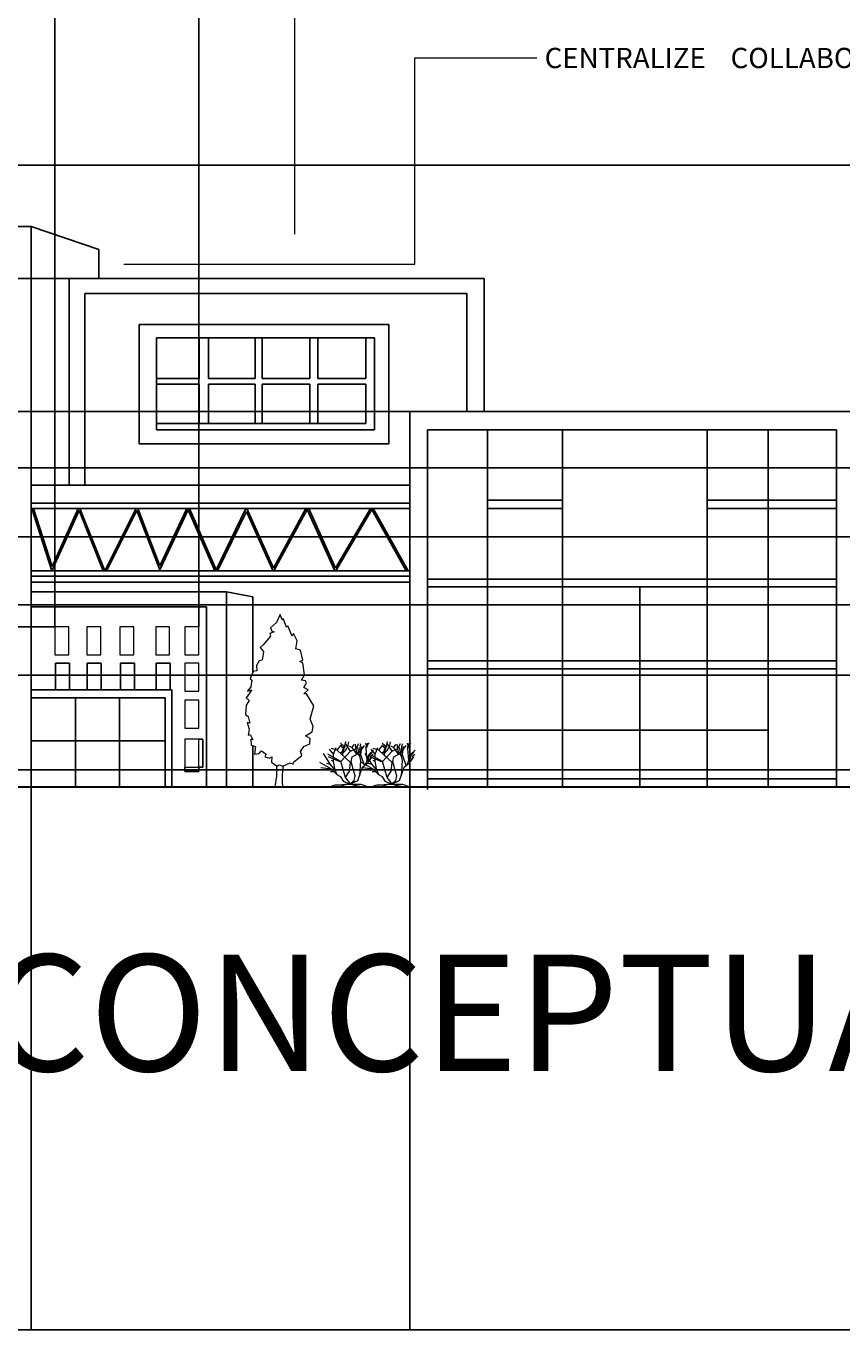
# Model space of a CAD drawing. Units: inches. Extents: x -32109 to 33221, y -19197 to 7608.
# Tile 12 of 25: x -5707 to -741, y -5430 to 2510. Entities that reach past the tile are written whole.
import ezdxf

# ---------------------------------------------------------------- set-up
doc = ezdxf.new("R2010")
doc.units = ezdxf.units.IN
doc.header["$MEASUREMENT"] = 0
for name, color, linetype, lineweight in [('A-ANNO-DIMS', 2, 'Continuous', 18), ('A-ANNO-NOTE', 2, 'Continuous', 18), ('A-ANNO-TEXT', 7, 'Continuous', 25), ('A-ELEV', 7, 'Continuous', 25), ('A-GLAZ', 4, 'Continuous', 18), ('L-PLNT', 3, 'Continuous', 13)]:
    doc.layers.add(name, color=color, linetype=linetype, lineweight=lineweight)
doc.styles.get("Standard").update_dxf_attribs({"font": 'arial.ttf'})
doc.dimstyles.get("Standard").update_dxf_attribs({"dimtxt": 0.18, "dimasz": 0.18, "dimexe": 0.18, "dimexo": 0.0625, "dimgap": 0.09, "dimtad": 0, "dimtih": 1, "dimtoh": 1, "dimdec": 4, "dimzin": 0, "dimdsep": 46, "dimtxsty": 'Standard', "dimcen": 0.09, "dimadec": 0, "dimazin": 0, "dimtfac": 1, "dimtdec": 4, "dimtofl": 0, "dimtmove": 0, "dimatfit": 3, "dimfxl": 1, "dimtolj": 1, "dimtzin": 0, "dimarcsym": 0})

# ---------------------------------------------------------------- blocks, each defined once
blk = doc.blocks.new('*U2')
blk.add_lwpolyline([(-2.754, 191.699), (-6.78, 182.851), (-13.682, 176.953), (-11.956, 173.266), (-9.656, 172.529), (-14.257, 170.317), (-13.682, 167.368), (-21.733, 157.783), (-25.184, 154.834), (-21.158, 150.41), (-21.733, 147.461), (-22.884, 140.825), (-26.334, 140.087), (-29.21, 134.926), (-28.635, 129.028), (-32.661, 128.291), (-36.111, 120.18), (-34.386, 118.706), (-35.536, 111.333), (-38.987, 106.171), (-34.386, 107.646), (-40.712, 98.798), (-37.261, 95.849), (-40.712, 90.688), (-41.287, 80.366), (-38.412, 78.154), (-36.686, 70.781), (-39.562, 71.518), (-37.261, 64.145), (-38.412, 57.509), (-36.111, 58.247), (-33.236, 52.348), (-35.536, 53.086), (-34.961, 46.45), (-30.36, 44.975), (-31.51, 36.128), (-26.334, 36.865), (-23.459, 39.814), (-18.283, 36.128), (-20.008, 33.178), (-14.832, 31.704), (-11.956, 33.178), (-12.531, 27.28), (-6.205, 22.856), (-3.905, 24.331), (0.121, 22.856), (8.173, 26.543), (11.624, 25.068), (12.199, 27.28), (21.4, 34.653), (19.675, 39.077), (23.701, 44.975), (30.027, 47.924), (30.602, 53.823), (25.426, 56.772), (32.903, 61.196), (34.053, 67.094), (30.602, 75.205), (34.628, 89.951), (26.576, 103.222), (23.701, 103.222), (28.302, 107.646), (23.701, 110.595), (26.576, 115.756), (25.426, 117.968), (20.825, 118.706), (24.276, 124.604), (22.551, 137.876), (19.1, 139.35), (22.551, 140.825), (19.675, 151.884), (14.499, 153.359), (16.224, 162.207), (12.199, 170.317), (10.473, 167.368), (5.872, 179.165), (4.147, 177.69), (0.696, 187.275), (-0.454, 185.8)], close=True)
for points in [[(-6.813, 23.669), (-6.813, 11.669), (-8.627, 0)], [(0.387, 23.669), (-0.576, 13.271), (-0.576, 3.686), (0, 0)]]:
    blk.add_lwpolyline(points)
blk = doc.blocks.new('*U3')
for p, q in [((-14.88, 18.24), (-12.96, 20.64)), ((-12.471, 19.775), (-12.898, 22.044)), ((-11.28, 19.619), (-12.104, 21.184)), ((-11.921, 18.836), (-10.64, 20.401)), ((-11.433, 18.289), (-10.457, 22.749)), ((-8.16, 17.76), (-10.56, 21.6)), ((-9.48, 19.775), (-8.992, 22.592)), ((-7.2, 19.68), (-8.64, 20.16)), ((-7.2, 19.68), (-6.24, 21.12)), ((-5.086, 17.741), (-5.513, 21.34)), ((-5.28, 19.2), (-3.84, 21.6)), ((-3.84, 16.8), (-0.96, 20.64)), ((-3.377, 18.602), (-2.888, 21.575)), ((-2.88, 15.84), (-2.4, 20.16)), ((-0.508, 21.888), (-0.081, 20.558)), ((-0.203, 19.149), (0.102, 21.34)), ((-0.142, 19.384), (0.59, 20.401)), ((-0.02, 20.01), (0.896, 21.105)), ((0.041, 20.714), (1.384, 22.044)), ((0.102, 21.34), (0.835, 21.888)), ((-18.24, 11.04), (-21.755, 16.655)), ((-12.96, 12.48), (-19.68, 16.32)), ((-13.92, 12.48), (-19.2, 14.88)), ((-16.8, 16.32), (-18.72, 18.72)), ((-14.88, 18.24), (-17.76, 19.2)), ((-16.8, 16.32), (-15.36, 19.68)), ((-16.8, 12.48), (-16.8, 16.32)), ((-8.16, 12), (-14.88, 18.24)), ((-13.325, 16.724), (-11.433, 18.289)), ((-12.96, 12.48), (-8.16, 17.76)), ((-11.677, 19.071), (-12.471, 19.775)), ((-12.043, 15.628), (-11.921, 18.836)), ((-11.982, 16.802), (-10.579, 18.054)), ((-10.579, 18.054), (-9.846, 19.697)), ((-8.16, 17.76), (-5.28, 19.2)), ((-7.68, 12.48), (-7.2, 14.88)), ((-4.8, 16.32), (-7.2, 19.68)), ((-7.2, 14.88), (-3.84, 16.8)), ((-3.377, 15.315), (-5.086, 17.819)), ((-2.88, 12.96), (-4.32, 19.68)), ((-2.766, 16.802), (-3.377, 18.602)), ((-0.96, 10.56), (-2.88, 15.84)), ((0.346, 13.203), (-0.203, 19.149)), ((0.346, 13.203), (1.323, 16.254)), ((0.96, 12), (1.44, 15.36)), ((0.96, 12), (2.88, 14.88)), ((1.323, 16.254), (3.642, 18.289)), ((1.44, 15.36), (2.88, 17.28)), ((1.92, 13.44), (2.4, 15.36)), ((2.4, 15.36), (3.36, 16.32)), ((-17.76, 8.64), (-23.663, 11.961)), ((-17.76, 8.64), (-23.128, 9.222)), ((-18.24, 11.04), (-20.16, 11.52)), ((-15.84, 8.16), (-18.24, 11.04)), ((-16.32, 7.2), (-18.24, 7.2)), ((-16.8, 12.48), (-17.76, 12.96)), ((-14.88, 5.76), (-17.76, 8.64)), ((-15.84, 8.16), (-16.8, 12.48)), ((-14.88, 5.76), (-15.84, 8.16)), ((-12.96, 12.48), (-13.92, 12.48)), ((-10.56, 4.32), (-12.96, 12.48)), ((-10.56, 4.32), (-8.64, 7.68)), ((-8.64, 7.68), (-8.16, 12)), ((-6.72, 8.64), (-7.68, 12.48)), ((-5.76, 5.28), (-6.72, 8.64)), ((-4.32, 2.88), (-1.92, 9.6)), ((-3.36, 5.28), (-2.88, 12.96)), ((-1.92, 9.6), (0.96, 12)), ((-0.48, 10.8), (0.346, 13.203)), ((-15.84, 0.48), (-17.76, 0)), ((-13.44, 0.48), (-15.84, 0.48)), ((-12.96, 4.8), (-14.88, 5.76)), ((-9.6, 0.96), (-13.44, 0.48)), ((-11.52, 2.4), (-12.96, 4.8)), ((-9.6, 0.96), (-12.96, 0)), ((-8.64, 0.96), (-11.52, 2.4)), ((-8.64, 1.92), (-10.56, 4.32)), ((-9.6, 0.96), (-7.68, 0.96)), ((-8.64, 0.96), (-4.32, 2.88)), ((-8.64, 0.96), (-6.24, 2.88)), ((-8.64, 0.96), (-8.64, 1.92)), ((-8.64, 0.96), (-2.88, 0.96)), ((-7.68, 0.96), (-6.24, 0.48)), ((-6.24, 2.88), (-5.76, 5.28)), ((-6.24, 0.48), (-3.36, 0)), ((-2.88, 0.96), (0, 0))]:
    blk.add_line(p, q)
blk = doc.blocks.new('WIN-SMALL-A')
for p, q in [((0, 169.6), (0, 0)), ((84.9, 169.6), (0, 169.6)), ((84.9, 0), (84.9, 169.6)), ((0, 0), (84.9, 0))]:
    blk.add_line(p, q)
blk = doc.blocks.new('*D6')
at = {"layer": 'A-ANNO-DIMS', "color": 0, "lineweight": -2, "transparency": 16777216}
for p, q in [((-4656.1, -1833.3), (-4630.5, -1833.3)), ((-4630.7, -1833.5), (-4630.7, -1917.9)), ((-4630.7, -2002.8), (-4630.7, -1918.3)), ((-4656.1, -2002.9), (-4630.5, -2002.9))]:
    blk.add_line(p, q, dxfattribs=at)
at = {"layer": 'A-ANNO-DIMS', "color": 0, "transparency": 16777216}
for points in [[(-4630.7, -1833.5), (-4630.7, -1833.5), (-4630.7, -1833.3)], [(-4630.7, -2002.8), (-4630.7, -2002.8), (-4630.7, -2002.9)]]:
    blk.add_solid(points, dxfattribs=at)
at = {"layer": 'Defpoints', "color": 0, "transparency": 16777216}
for p in [(-4656.1, -1833.3), (-4656.1, -2002.9), (-4630.7, -2002.9)]:
    blk.add_point(p, dxfattribs=at)
at = {"layer": 'A-ANNO-DIMS', "color": 0, "transparency": 16777216, "insert": (-4630.7, -1918.1), "char_height": 0.18, "attachment_point": 5}
blk.add_mtext('\\A1;SMALL WINDOW A 170 TYP.', dxfattribs=at)
blk = doc.blocks.new('*D7')
at = {"layer": 'A-ANNO-DIMS', "color": 0, "lineweight": -2, "transparency": 16777216}
for p, q in [((-4741.1, -2003), (-4741.1, -2028.6)), ((-4740.9, -2028.4), (-4699.1, -2028.4)), ((-4656.3, -2028.4), (-4698.1, -2028.4)), ((-4656.1, -2003), (-4656.1, -2028.6))]:
    blk.add_line(p, q, dxfattribs=at)
at = {"layer": 'A-ANNO-DIMS', "color": 0, "transparency": 16777216}
for points in [[(-4740.9, -2028.4), (-4740.9, -2028.4), (-4741.1, -2028.4)], [(-4656.3, -2028.4), (-4656.3, -2028.4), (-4656.1, -2028.4)]]:
    blk.add_solid(points, dxfattribs=at)
at = {"layer": 'Defpoints', "color": 0, "transparency": 16777216}
for p in [(-4741.1, -2002.9), (-4741.1, -2028.4), (-4656.1, -2002.9)]:
    blk.add_point(p, dxfattribs=at)
at = {"layer": 'A-ANNO-DIMS', "color": 0, "transparency": 16777216, "insert": (-4698.6, -2028.4), "char_height": 0.18, "attachment_point": 5}
blk.add_mtext('\\A1;85 TYP.', dxfattribs=at)
blk = doc.blocks.new('*D10')
at = {"layer": 'A-ANNO-DIMS', "color": 0, "lineweight": -2, "transparency": 16777216}
for p, q in [((-18512.6, -110.2), (-18512.6, 5772)), ((-18512.5, 5771.8), (-202.1, 5771.8)), ((18109.1, 5771.8), (-201.2, 5771.8)), ((18109.3, -101.5), (18109.3, 5772))]:
    blk.add_line(p, q, dxfattribs=at)
at = {"layer": 'A-ANNO-DIMS', "color": 0, "transparency": 16777216}
for points in [[(-18512.5, 5771.9), (-18512.5, 5771.8), (-18512.6, 5771.8)], [(18109.1, 5771.9), (18109.1, 5771.8), (18109.3, 5771.8)]]:
    blk.add_solid(points, dxfattribs=at)
at = {"layer": 'Defpoints', "color": 0, "transparency": 16777216}
for p in [(18109.3, 5771.8), (-18512.6, -110.2), (18109.3, -101.6)]:
    blk.add_point(p, dxfattribs=at)
at = {"layer": 'A-ANNO-DIMS', "color": 0, "transparency": 16777216, "insert": (-201.7, 5771.8), "char_height": 0.18, "attachment_point": 5}
blk.add_mtext('\\A1;36622', dxfattribs=at)
blk = doc.blocks.new('*D11')
at = {"layer": 'A-ANNO-DIMS', "color": 0, "lineweight": -2, "transparency": 16777216}
for p, q in [((14509.6, 1705.2), (25710.6, 1705.2)), ((25710.5, 1705), (25710.5, -209.6)), ((25710.5, -2124.6), (25710.5, -210)), ((-18512.6, -2124.8), (25710.6, -2124.8))]:
    blk.add_line(p, q, dxfattribs=at)
at = {"layer": 'A-ANNO-DIMS', "color": 0, "transparency": 16777216}
for points in [[(25710.4, 1705), (25710.5, 1705), (25710.5, 1705.2)], [(25710.4, -2124.6), (25710.5, -2124.6), (25710.5, -2124.8)]]:
    blk.add_solid(points, dxfattribs=at)
at = {"layer": 'Defpoints', "color": 0, "transparency": 16777216}
for p in [(14509.6, 1705.2), (-18512.6, -2124.8), (25710.5, -2124.8)]:
    blk.add_point(p, dxfattribs=at)
at = {"layer": 'A-ANNO-DIMS', "color": 0, "transparency": 16777216, "insert": (25710.5, -209.8), "char_height": 0.18, "attachment_point": 5}
blk.add_mtext('\\A1;3830', dxfattribs=at)
blk = doc.blocks.new('*D20')
at = {"layer": 'A-ANNO-DIMS', "color": 0, "lineweight": -2, "transparency": 16777216}
for p, q in [((-5532.1, -1149.2), (-5532.1, 5772)), ((-5531.9, 5771.8), (-5094.4, 5771.8)), ((-4656.3, 5771.8), (-5093.8, 5771.8)), ((-4656.1, -1149.2), (-4656.1, 5772))]:
    blk.add_line(p, q, dxfattribs=at)
at = {"layer": 'A-ANNO-DIMS', "color": 0, "transparency": 16777216}
for points in [[(-5531.9, 5771.9), (-5531.9, 5771.8), (-5532.1, 5771.8)], [(-4656.3, 5771.9), (-4656.3, 5771.8), (-4656.1, 5771.8)]]:
    blk.add_solid(points, dxfattribs=at)
at = {"layer": 'Defpoints', "color": 0, "transparency": 16777216}
for p in [(-4656.1, 5771.8), (-5532.1, -1149.2), (-4656.1, -1149.2)]:
    blk.add_point(p, dxfattribs=at)
at = {"layer": 'A-ANNO-DIMS', "color": 0, "transparency": 16777216, "insert": (-5094.1, 5771.8), "char_height": 0.18, "attachment_point": 5}
blk.add_mtext('\\A1;876', dxfattribs=at)
blk = doc.blocks.new('*D21')
at = {"layer": 'A-ANNO-DIMS', "color": 0, "lineweight": -2, "transparency": 16777216}
for p, q in [((-5532.2, -1149.2), (-24362, -1149.2)), ((-24361.8, -1149.4), (-24361.8, -1636.8)), ((-24361.8, -2124.6), (-24361.8, -1637.2)), ((-5677.1, -2124.8), (-24362, -2124.8))]:
    blk.add_line(p, q, dxfattribs=at)
at = {"layer": 'A-ANNO-DIMS', "color": 0, "transparency": 16777216}
for points in [[(-24361.8, -1149.4), (-24361.8, -1149.4), (-24361.8, -1149.2)], [(-24361.8, -2124.6), (-24361.8, -2124.6), (-24361.8, -2124.8)]]:
    blk.add_solid(points, dxfattribs=at)
at = {"layer": 'Defpoints', "color": 0, "transparency": 16777216}
for p in [(-24361.8, -1149.2), (-5532.1, -1149.2), (-5677.1, -2124.8)]:
    blk.add_point(p, dxfattribs=at)
at = {"layer": 'A-ANNO-DIMS', "color": 0, "transparency": 16777216, "insert": (-24361.8, -1637), "char_height": 0.18, "attachment_point": 5}
blk.add_mtext('\\A1;975.6', dxfattribs=at)
blk = doc.blocks.new('*D29')
at = {"layer": 'A-ANNO-DIMS', "color": 0, "lineweight": -2, "transparency": 16777216}
for p, q in [((-7754.4, -2118.5), (-7754.4, -5429.7)), ((-5677.1, -2124.9), (-5677.1, -5429.7)), ((-7754.2, -5429.6), (-6716.2, -5429.6)), ((-5677.3, -5429.6), (-6715.3, -5429.6))]:
    blk.add_line(p, q, dxfattribs=at)
at = {"layer": 'A-ANNO-DIMS', "color": 0, "transparency": 16777216}
for points in [[(-7754.2, -5429.5), (-7754.2, -5429.6), (-7754.4, -5429.6)], [(-5677.3, -5429.5), (-5677.3, -5429.6), (-5677.1, -5429.6)]]:
    blk.add_solid(points, dxfattribs=at)
at = {"layer": 'Defpoints', "color": 0, "transparency": 16777216}
for p in [(-7754.4, -2118.4), (-5677.1, -2124.8), (-5677.1, -5429.6)]:
    blk.add_point(p, dxfattribs=at)
at = {"layer": 'A-ANNO-DIMS', "color": 0, "transparency": 16777216, "insert": (-6715.7, -5429.6), "char_height": 0.18, "attachment_point": 5}
blk.add_mtext('\\A1;2077.3', dxfattribs=at)
blk = doc.blocks.new('*D30')
at = {"layer": 'A-ANNO-DIMS', "color": 0, "lineweight": -2, "transparency": 16777216}
for p, q in [((-5677.1, -2124.9), (-5677.1, -5429.7)), ((-3370.6, -2124.9), (-3370.6, -5429.7)), ((-5676.9, -5429.6), (-4524.3, -5429.6)), ((-3370.7, -5429.6), (-4523.4, -5429.6))]:
    blk.add_line(p, q, dxfattribs=at)
at = {"layer": 'A-ANNO-DIMS', "color": 0, "transparency": 16777216}
for points in [[(-5676.9, -5429.5), (-5676.9, -5429.6), (-5677.1, -5429.6)], [(-3370.7, -5429.5), (-3370.7, -5429.6), (-3370.6, -5429.6)]]:
    blk.add_solid(points, dxfattribs=at)
at = {"layer": 'Defpoints', "color": 0, "transparency": 16777216}
for p in [(-5677.1, -2124.8), (-3370.6, -2124.8), (-3370.6, -5429.6)]:
    blk.add_point(p, dxfattribs=at)
at = {"layer": 'A-ANNO-DIMS', "color": 0, "transparency": 16777216, "insert": (-4523.8, -5429.6), "char_height": 0.18, "attachment_point": 5}
blk.add_mtext('\\A1;2306.5', dxfattribs=at)
blk = doc.blocks.new('*D31')
at = {"layer": 'A-ANNO-DIMS', "color": 0, "lineweight": -2, "transparency": 16777216}
for p, q in [((-3370.6, -2124.9), (-3370.6, -5429.7)), ((-651, -2124.9), (-651, -5429.7)), ((-3370.4, -5429.6), (-2011.2, -5429.6)), ((-651.1, -5429.6), (-2010.3, -5429.6))]:
    blk.add_line(p, q, dxfattribs=at)
at = {"layer": 'A-ANNO-DIMS', "color": 0, "transparency": 16777216}
for points in [[(-3370.4, -5429.5), (-3370.4, -5429.6), (-3370.6, -5429.6)], [(-651.1, -5429.5), (-651.1, -5429.6), (-651, -5429.6)]]:
    blk.add_solid(points, dxfattribs=at)
at = {"layer": 'Defpoints', "color": 0, "transparency": 16777216}
for p in [(-3370.6, -2124.8), (-651, -2124.8), (-651, -5429.6)]:
    blk.add_point(p, dxfattribs=at)
at = {"layer": 'A-ANNO-DIMS', "color": 0, "transparency": 16777216, "insert": (-2010.8, -5429.6), "char_height": 0.18, "attachment_point": 5}
blk.add_mtext('\\A1;2719.6', dxfattribs=at)
blk = doc.blocks.new('*D40')
at = {"layer": 'A-ANNO-DIMS', "color": 0, "lineweight": -2, "transparency": 16777216}
for p, q in [((-5445.1, 973), (-24362, 973)), ((-24361.8, 972.8), (-24361.8, -575.7)), ((-24361.8, -2124.6), (-24361.8, -576.1)), ((-5677.1, -2124.8), (-24362, -2124.8))]:
    blk.add_line(p, q, dxfattribs=at)
at = {"layer": 'A-ANNO-DIMS', "color": 0, "transparency": 16777216}
for points in [[(-24361.8, 972.8), (-24361.8, 972.8), (-24361.8, 973)], [(-24361.8, -2124.6), (-24361.8, -2124.6), (-24361.8, -2124.8)]]:
    blk.add_solid(points, dxfattribs=at)
at = {"layer": 'Defpoints', "color": 0, "transparency": 16777216}
for p in [(-5445, 973), (-24361.8, -2124.8), (-5677.1, -2124.8)]:
    blk.add_point(p, dxfattribs=at)
at = {"layer": 'A-ANNO-DIMS', "color": 0, "transparency": 16777216, "insert": (-24361.8, -575.9), "char_height": 0.18, "attachment_point": 5}
blk.add_mtext('\\A1;3098', dxfattribs=at)
blk = doc.blocks.new('*D41')
at = {"layer": 'A-ANNO-DIMS', "color": 0, "lineweight": -2, "transparency": 16777216}
for p, q in [((-651, 162.2), (-24362, 162.2)), ((-24361.8, 162), (-24361.8, -981.1)), ((-24361.8, -2124.6), (-24361.8, -981.5)), ((-651, -2124.8), (-24362, -2124.8))]:
    blk.add_line(p, q, dxfattribs=at)
at = {"layer": 'A-ANNO-DIMS', "color": 0, "transparency": 16777216}
for points in [[(-24361.8, 162), (-24361.8, 162), (-24361.8, 162.2)], [(-24361.8, -2124.6), (-24361.8, -2124.6), (-24361.8, -2124.8)]]:
    blk.add_solid(points, dxfattribs=at)
at = {"layer": 'Defpoints', "color": 0, "transparency": 16777216}
for p in [(-651, 162.2), (-24361.8, -2124.8), (-651, -2124.8)]:
    blk.add_point(p, dxfattribs=at)
at = {"layer": 'A-ANNO-DIMS', "color": 0, "transparency": 16777216, "insert": (-24361.8, -981.3), "char_height": 0.18, "attachment_point": 5}
blk.add_mtext('\\A1;2287', dxfattribs=at)
blk = doc.blocks.new('*D53')
at = {"layer": 'A-ANNO-DIMS', "color": 0, "lineweight": -2, "transparency": 16777216}
for p, q in [((-9508.3, -179.7), (25710.6, -179.7)), ((25710.5, -179.9), (25710.5, -389.7)), ((25710.5, -600), (25710.5, -390.1)), ((-9508.3, -600.2), (25710.6, -600.2))]:
    blk.add_line(p, q, dxfattribs=at)
at = {"layer": 'A-ANNO-DIMS', "color": 0, "transparency": 16777216}
for points in [[(25710.4, -179.9), (25710.5, -179.9), (25710.5, -179.7)], [(25710.4, -600), (25710.5, -600), (25710.5, -600.2)]]:
    blk.add_solid(points, dxfattribs=at)
at = {"layer": 'Defpoints', "color": 0, "transparency": 16777216}
for p in [(-9508.3, -179.7), (-9508.3, -600.2), (25710.5, -600.2)]:
    blk.add_point(p, dxfattribs=at)
at = {"layer": 'A-ANNO-DIMS', "color": 0, "transparency": 16777216, "insert": (25710.5, -389.9), "char_height": 0.18, "attachment_point": 5}
blk.add_mtext('\\A1;420.5', dxfattribs=at)
blk = doc.blocks.new('*D54')
at = {"layer": 'A-ANNO-DIMS', "color": 0, "lineweight": -2, "transparency": 16777216}
for p, q in [((-9508.3, -600.2), (25710.6, -600.2)), ((25710.5, -600.3), (25710.5, -806.8)), ((25710.5, -1013.7), (25710.5, -807.2)), ((-9508.3, -1013.9), (25710.6, -1013.9))]:
    blk.add_line(p, q, dxfattribs=at)
at = {"layer": 'A-ANNO-DIMS', "color": 0, "transparency": 16777216}
for points in [[(25710.4, -600.3), (25710.5, -600.3), (25710.5, -600.2)], [(25710.4, -1013.7), (25710.5, -1013.7), (25710.5, -1013.9)]]:
    blk.add_solid(points, dxfattribs=at)
at = {"layer": 'Defpoints', "color": 0, "transparency": 16777216}
for p in [(-9508.3, -600.2), (-9508.3, -1013.9), (25710.5, -1013.9)]:
    blk.add_point(p, dxfattribs=at)
at = {"layer": 'A-ANNO-DIMS', "color": 0, "transparency": 16777216, "insert": (25710.5, -807), "char_height": 0.18, "attachment_point": 5}
blk.add_mtext('\\A1;413.7', dxfattribs=at)
blk = doc.blocks.new('*D55')
at = {"layer": 'A-ANNO-DIMS', "color": 0, "lineweight": -2, "transparency": 16777216}
for p, q in [((-9508.3, -1013.9), (25710.6, -1013.9)), ((25710.5, -1014.1), (25710.5, -1227.7)), ((25710.5, -1441.6), (25710.5, -1228)), ((-9508.3, -1441.8), (25710.6, -1441.8))]:
    blk.add_line(p, q, dxfattribs=at)
at = {"layer": 'A-ANNO-DIMS', "color": 0, "transparency": 16777216}
for points in [[(25710.4, -1014.1), (25710.5, -1014.1), (25710.5, -1013.9)], [(25710.4, -1441.6), (25710.5, -1441.6), (25710.5, -1441.8)]]:
    blk.add_solid(points, dxfattribs=at)
at = {"layer": 'Defpoints', "color": 0, "transparency": 16777216}
for p in [(-9508.3, -1013.9), (-9508.3, -1441.8), (25710.5, -1441.8)]:
    blk.add_point(p, dxfattribs=at)
at = {"layer": 'A-ANNO-DIMS', "color": 0, "transparency": 16777216, "insert": (25710.5, -1227.9), "char_height": 0.18, "attachment_point": 5}
blk.add_mtext('\\A1;427.9', dxfattribs=at)
blk = doc.blocks.new('*D56')
at = {"layer": 'A-ANNO-DIMS', "color": 0, "lineweight": -2, "transparency": 16777216}
for p, q in [((-9508.3, -1441.8), (25710.6, -1441.8)), ((25710.5, -1442), (25710.5, -1730.1)), ((25710.5, -2018.6), (25710.5, -1730.5)), ((-9508.3, -2018.8), (25710.6, -2018.8))]:
    blk.add_line(p, q, dxfattribs=at)
at = {"layer": 'A-ANNO-DIMS', "color": 0, "transparency": 16777216}
for points in [[(25710.4, -1442), (25710.5, -1442), (25710.5, -1441.8)], [(25710.4, -2018.6), (25710.5, -2018.6), (25710.5, -2018.8)]]:
    blk.add_solid(points, dxfattribs=at)
at = {"layer": 'Defpoints', "color": 0, "transparency": 16777216}
for p in [(-9508.3, -1441.8), (-9508.3, -2018.8), (25710.5, -2018.8)]:
    blk.add_point(p, dxfattribs=at)
at = {"layer": 'A-ANNO-DIMS', "color": 0, "transparency": 16777216, "insert": (25710.5, -1730.3), "char_height": 0.18, "attachment_point": 5}
blk.add_mtext('\\A1;576.9', dxfattribs=at)
blk = doc.blocks.new('*D158')
at = {"layer": 'A-ANNO-DIMS', "color": 0, "lineweight": -2, "transparency": 16777216}
for p, q in [((5447.3, 1662.2), (-24362, 1662.2)), ((-24361.8, 1662), (-24361.8, -230.1)), ((-24361.8, -2122.6), (-24361.8, -230.5)), ((5279.2, -2122.7), (-24362, -2122.7))]:
    blk.add_line(p, q, dxfattribs=at)
at = {"layer": 'A-ANNO-DIMS', "color": 0, "transparency": 16777216}
for points in [[(-24361.8, 1662), (-24361.8, 1662), (-24361.8, 1662.2)], [(-24361.8, -2122.6), (-24361.8, -2122.6), (-24361.8, -2122.7)]]:
    blk.add_solid(points, dxfattribs=at)
at = {"layer": 'Defpoints', "color": 0, "transparency": 16777216}
for p in [(5447.3, 1662.2), (-24361.8, -2122.7), (5279.3, -2122.7)]:
    blk.add_point(p, dxfattribs=at)
at = {"layer": 'A-ANNO-DIMS', "color": 0, "transparency": 16777216, "insert": (-24361.8, -230.3), "char_height": 0.18, "attachment_point": 5}
blk.add_mtext('\\A1;3784.9', dxfattribs=at)

msp = doc.modelspace()

# ---------------------------------------------------------------- linework, layer by layer
at = {"layer": 'A-ANNO-NOTE'}
for p, q in [((-4070.256, 1242.026), (-4070.256, 3321.835)), ((-3340.327, 1059.41), (-3340.327, 2317.456)), ((-3340.327, 2317.456), (-2597.229, 2317.456)), ((-5112.618, 1059.41), (-3340.327, 1059.41))]:
    msp.add_line(p, q, dxfattribs=at)
at = {"layer": 'A-ELEV'}
for p, q in [((-5677.079, 1290.029), (-7375.878, 1290.029)), ((-5677.079, 705.707), (-5677.079, 1290.029)), ((-5677.079, 1290.029), (-5264.468, 1149.061)), ((-5264.468, 973.011), (-5264.468, 1149.061)), ((-5445.024, 973.011), (-2919.008, 973.011)), ((-5445.024, 973.011), (-5445.024, -286.113)), ((-2919.008, 973.011), (-2919.008, 162.186)), ((-5350.049, -286.113), (-5350.049, 880.414)), ((-5350.049, 880.414), (-3024.183, 880.414)), ((-3024.183, 880.414), (-3024.183, 162.186)), ((-5677.079, 705.707), (-5677.079, 115.673)), ((-5019.261, 693.125), (-3498.949, 693.125)), ((-5019.261, 693.125), (-5019.261, -33.953)), ((-3498.949, 693.125), (-3498.949, -33.953)), ((-4914.008, 611.561), (-3585.505, 611.561)), ((-4914.008, 51.166), (-4914.008, 611.561)), ((-4652.588, 364.767), (-4652.588, 611.561)), ((-4595.774, 364.767), (-4595.774, 611.561)), ((-4313.328, 364.767), (-4313.328, 611.561)), ((-4270.84, 364.767), (-4270.84, 611.561)), ((-3978.939, 364.767), (-3978.939, 611.561)), ((-3930.362, 364.767), (-3930.362, 611.561)), ((-3638.056, 364.767), (-3638.056, 611.561)), ((-3585.505, 611.561), (-3585.505, 51.166)), ((-4914.008, 364.767), (-4652.588, 364.767)), ((-4914.008, 329.958), (-4652.588, 329.958)), ((-4652.588, 90.392), (-4652.588, 329.958)), ((-4595.774, 364.767), (-4313.328, 364.767)), ((-4595.774, 90.392), (-4595.774, 329.958)), ((-4595.774, 329.958), (-4313.328, 329.958)), ((-4313.328, 90.392), (-4313.328, 329.958)), ((-4270.84, 364.767), (-3978.939, 364.767)), ((-4270.84, 90.392), (-4270.84, 329.958)), ((-4270.84, 329.958), (-3978.939, 329.958)), ((-3978.939, 90.392), (-3978.939, 329.958)), ((-3930.362, 364.767), (-3638.056, 364.767)), ((-3930.362, 90.392), (-3930.362, 329.958)), ((-3930.362, 329.958), (-3638.056, 329.958)), ((-3638.056, 90.392), (-3638.056, 329.958)), ((-3370.568, 162.186), (-3370.568, -2124.791)), ((-3370.568, 162.186), (-650.959, 162.186)), ((-5677.079, -332.626), (-5677.079, 115.673)), ((-4914.008, 90.392), (-3638.056, 90.392)), ((-3585.505, 51.166), (-4914.008, 51.166)), ((-3264.186, -2138.615), (-3264.186, 50.575)), ((-3264.186, 50.575), (-773.951, 50.575)), ((-2897.717, -2124.791), (-2897.717, 50.575)), ((-2441.631, -2124.791), (-2441.631, 50.575)), ((-1560.381, -2124.791), (-1560.381, 50.575)), ((-1189.328, -2124.791), (-1189.328, 50.575)), ((-773.951, 50.575), (-773.951, -2124.791)), ((-5019.261, -33.953), (-3498.949, -33.953)), ((-3370.568, -286.113), (-5677.079, -286.113)), ((-5677.079, -332.626), (-5677.079, -830.732)), ((-5677.079, -391.831), (-5677.079, -2124.791)), ((-3370.568, -395.582), (-5677.079, -395.582)), ((-5677.079, -428.305), (-5677.079, -395.582)), ((-2897.717, -376.671), (-2441.631, -376.671)), ((-1560.381, -376.671), (-773.951, -376.671)), ((-3370.568, -428.305), (-5677.079, -428.305)), ((-5551.082, -807.889), (-5671.515, -428.405)), ((-5548.872, -781.794), (-5661.055, -428.305)), ((-5384.649, -440.748), (-5549.635, -807.889)), ((-5390.021, -428.305), (-5548.872, -781.794)), ((-5238.795, -807.889), (-5384.649, -440.748)), ((-5228.035, -807.889), (-5378.938, -428.039)), ((-5037.846, -428.305), (-5228.035, -807.889)), ((-5032.966, -440.89), (-5216.85, -807.889)), ((-4893.037, -801.767), (-5032.966, -440.89)), ((-4892.141, -776.417), (-5027.121, -428.305)), ((-4720.655, -436.159), (-4893.037, -801.767)), ((-4728.008, -428.305), (-4892.141, -776.417)), ((-4558.37, -807.889), (-4720.655, -436.159)), ((-4550.131, -801.767), (-4713.172, -428.305)), ((-4368.579, -428.305), (-4550.131, -801.767)), ((-4365.883, -445.631), (-4541.988, -807.889)), ((-4205.368, -805.837), (-4365.883, -445.631)), ((-4201.36, -790.264), (-4362.655, -428.305)), ((-4004.453, -428.305), (-4201.36, -790.264)), ((-3995.61, -432.976), (-4199.564, -807.889)), ((-3826.957, -807.38), (-3995.61, -432.976)), ((-3822.889, -792.063), (-3986.746, -428.305)), ((-3611.41, -428.305), (-3822.889, -792.063)), ((-3602.51, -432.894), (-3820.522, -807.889)), ((-3393.349, -807.889), (-3602.51, -432.894)), ((-3381.898, -807.889), (-3593.619, -428.305)), ((-2897.717, -427.797), (-2441.631, -427.797)), ((-1560.381, -427.797), (-773.951, -427.797)), ((-5644.503, -807.889), (-5677.079, -807.889)), ((-5644.503, -840.13), (-5677.079, -840.13)), ((-3370.568, -807.889), (-5644.503, -807.889)), ((-5644.503, -840.13), (-3370.568, -840.13)), ((-3264.186, -857.34), (-773.951, -857.34)), ((-3370.568, -876.961), (-5677.079, -876.961)), ((-5677.079, -936.121), (-4487.327, -936.121)), ((-4487.327, -936.121), (-4487.327, -2124.791)), ((-4487.327, -936.121), (-4327.564, -966.442)), ((-3264.186, -905.626), (-773.951, -905.626)), ((-1970.085, -2124.791), (-1970.085, -905.626)), ((-4608.001, -1027.184), (-5677.079, -1027.184)), ((-4608.001, -2124.791), (-4608.001, -1027.184)), ((-4327.564, -966.442), (-4327.564, -1428.724)), ((-5527.29, -1369.774), (-5527.29, -1532.969)), ((-5442.363, -1369.774), (-5527.29, -1369.774)), ((-5442.363, -1532.969), (-5442.363, -1369.774)), ((-5335.598, -1369.774), (-5335.598, -1532.969)), ((-5250.672, -1369.774), (-5335.598, -1369.774)), ((-5250.672, -1532.969), (-5250.672, -1369.774)), ((-5131.775, -1369.774), (-5131.775, -1532.969)), ((-5046.848, -1369.774), (-5131.775, -1369.774)), ((-5046.848, -1532.969), (-5046.848, -1369.774)), ((-4915.819, -1369.774), (-4915.819, -1532.969)), ((-4830.893, -1369.774), (-4915.819, -1369.774)), ((-4830.893, -1532.969), (-4830.893, -1369.774)), ((-3264.186, -1355.427), (-773.951, -1355.427)), ((-3264.186, -1403.713), (-773.951, -1403.713)), ((-4820.848, -1532.969), (-5677.079, -1532.969)), ((-4861.31, -1580.706), (-5677.079, -1580.706)), ((-5406.64, -1580.706), (-5406.64, -2124.791)), ((-5138.567, -1580.706), (-5138.567, -2124.791)), ((-4861.31, -2124.791), (-4861.31, -1580.706)), ((-4820.848, -2116.472), (-4820.848, -1532.969)), ((-3264.186, -1776.697), (-1189.328, -1776.697)), ((-4861.31, -1842.995), (-5677.079, -1842.995)), ((-4327.564, -1834.563), (-4327.564, -1835.544)), ((-4327.564, -1870.859), (-4327.564, -2124.791)), ((-18512.647, -2124.791), (1683.588, -2124.791)), ((-3437.624, -2124.791), (-10277.124, -2124.791)), ((-5677.079, -2124.791), (-5737.208, -2124.791)), ((-4487.327, -2124.791), (-4608.001, -2124.791)), ((-3264.186, -2074.934), (-773.951, -2074.934))]:
    msp.add_line(p, q, dxfattribs=at)

# ---------------------------------------------------------------- block references
at = {"layer": 'A-GLAZ'}
msp.add_blockref('WIN-SMALL-A', (-5532.101, -1318.879), dxfattribs=at)
at = {"layer": 'A-GLAZ', "rotation": 180}
for p in [(-5253.057, -1149.23), (-5051.66, -1149.23), (-4833.278, -1149.23), (-4656.145, -1149.23), (-4656.145, -1369.774), (-4656.145, -1595.783), (-4656.145, -1833.292)]:
    msp.add_blockref('WIN-SMALL-A', p, dxfattribs=at)
at = {"layer": 'L-PLNT'}
for name, p, xscale, yscale, zscale in [('*U2', (-4145.053, -2122.295), 5.474302449835042, 5.474302449835042, 5.474302449835042), ('*U3', (-3635.267, -2118.431), 11.97885450539613, 11.97885450539613, 11.97885450539613), ('*U3', (-3381.756, -2118.431), 11.97885450539613, 11.97885450539613, 11.97885450539613)]:
    msp.add_blockref(name, p, dxfattribs=dict(at, xscale=xscale, yscale=yscale, zscale=zscale))

# ---------------------------------------------------------------- texts
at = {"layer": 'A-ANNO-TEXT'}
for s, height, p in [('CENTRALIZE    COLLABORATION   HUB', 123.55474, (-2550.352, 2253.723)), ('MONUMENTAL    FRONT   FACADE    ( CONCEPTUAL ONLY   NO DIMENSIONS )', 709.79495, (-22238.107, -3853.852))]:
    msp.add_text(s, height=height, dxfattribs=at).set_placement(p)

# ---------------------------------------------------------------- dimensions: what is measured, and where the dimension line sits
at = {"layer": 'A-ANNO-DIMS'}
for base, p1, p2, override, picture, middle in [((18109.317, 5771.835), (-18512.647, -110.242), (18109.317, -101.6), {"dimdec": 0, "dimlfac": 1, "dimrnd": 0, "dimzin": 0, "dimdsep": 46, "dimlunit": 2}, '*D10', (-201.665, 5771.835)), ((-4656.145, 5771.835), (-5532.101, -1149.23), (-4656.145, -1149.23), {"dimdec": 0, "dimlfac": 1, "dimrnd": 0, "dimzin": 0, "dimdsep": 46, "dimlunit": 2}, '*D20', (-5094.123, 5771.835)), ((-5677.079, -5429.555), (-7754.412, -2118.431), (-5677.079, -2124.791), {"dimdec": 1, "dimlfac": 1, "dimrnd": 0, "dimzin": 0, "dimdsep": 46, "dimlunit": 2}, '*D29', (-6715.746, -5429.555)), ((-3370.568, -5429.555), (-5677.079, -2124.791), (-3370.568, -2124.791), {"dimdec": 1, "dimlfac": 1, "dimrnd": 0, "dimzin": 0, "dimdsep": 46, "dimlunit": 2}, '*D30', (-4523.824, -5429.555)), ((-650.959, -5429.555), (-3370.568, -2124.791), (-650.959, -2124.791), {"dimdec": 1, "dimlfac": 1, "dimrnd": 0, "dimzin": 0, "dimdsep": 46, "dimlunit": 2}, '*D31', (-2010.764, -5429.555))]:
    dim = msp.add_linear_dim(base=base, p1=p1, p2=p2, dimstyle='Standard', override=override, dxfattribs=at)
    dim.commit()
    dim.dimension.update_dxf_attribs({"geometry": picture, "text_midpoint": middle})
for base, p1, p2, override, picture, middle in [((25710.469, -2124.791), (14509.55, 1705.162), (-18512.647, -2124.791), {"dimdec": 0, "dimlfac": 1, "dimrnd": 0, "dimzin": 0, "dimdsep": 46, "dimlunit": 2}, '*D11', (25710.469, -209.814)), ((-24361.816, -2122.749), (5447.329, 1662.17), (5279.264, -2122.749), {"dimdec": 1, "dimlfac": 1, "dimrnd": 0, "dimzin": 0, "dimdsep": 46, "dimlunit": 2}, '*D158', (-24361.816, -230.29)), ((-24361.816, -2124.791), (-5445.024, 973.011), (-5677.079, -2124.791), {"dimdec": 0, "dimlfac": 1, "dimrnd": 0, "dimzin": 0, "dimdsep": 46, "dimlunit": 2}, '*D40', (-24361.816, -575.89)), ((-24361.816, -2124.791), (-650.959, 162.186), (-650.959, -2124.791), {"dimdec": 0, "dimlfac": 1, "dimrnd": 0, "dimzin": 0, "dimdsep": 46, "dimlunit": 2}, '*D41', (-24361.816, -981.302)), ((25710.469, -600.154), (-9508.333, -179.679), (-9508.333, -600.154), {"dimdec": 1, "dimlfac": 1, "dimrnd": 0, "dimzin": 0, "dimdsep": 46, "dimlunit": 2}, '*D53', (25710.469, -389.916)), ((25710.469, -1013.888), (-9508.333, -600.154), (-9508.333, -1013.888), {"dimdec": 1, "dimlfac": 1, "dimrnd": 0, "dimzin": 0, "dimdsep": 46, "dimlunit": 2}, '*D54', (25710.469, -807.021)), ((25710.469, -1441.815), (-9508.333, -1013.888), (-9508.333, -1441.815), {"dimdec": 1, "dimlfac": 1, "dimrnd": 0, "dimzin": 0, "dimdsep": 46, "dimlunit": 2}, '*D55', (25710.469, -1227.851)), ((-24361.816, -1149.23), (-5677.079, -2124.791), (-5532.101, -1149.23), {"dimdec": 1, "dimlfac": 1, "dimrnd": 0, "dimzin": 0, "dimdsep": 46, "dimlunit": 2}, '*D21', (-24361.816, -1637.01)), ((25710.469, -2018.754), (-9508.333, -1441.815), (-9508.333, -2018.754), {"dimdec": 1, "dimlfac": 1, "dimrnd": 0, "dimzin": 0, "dimdsep": 46, "dimlunit": 2}, '*D56', (25710.469, -1730.285))]:
    dim = msp.add_linear_dim(base=base, p1=p1, p2=p2, angle=90, dimstyle='Standard', override=override, dxfattribs=at)
    dim.commit()
    dim.dimension.update_dxf_attribs({"geometry": picture, "text_midpoint": middle})
for base, p1, p2, angle, text, picture, middle in [((-4630.698, -2002.942), (-4656.145, -1833.292), (-4656.145, -2002.942), 270, 'SMALL WINDOW A <> TYP.', '*D6', (-4630.698, -1918.117)), ((-4741.072, -2028.389), (-4656.145, -2002.942), (-4741.072, -2002.942), 180, '<> TYP.', '*D7', (-4698.608, -2028.389))]:
    dim = msp.add_linear_dim(base=base, p1=p1, p2=p2, angle=angle, text=text, dimstyle='Standard', override={"dimdec": 0, "dimlfac": 1, "dimrnd": 0, "dimzin": 0, "dimdsep": 46, "dimlunit": 2}, dxfattribs=at)
    dim.commit()
    dim.dimension.update_dxf_attribs({"geometry": picture, "text_midpoint": middle})

doc.saveas('drawing.dxf')
